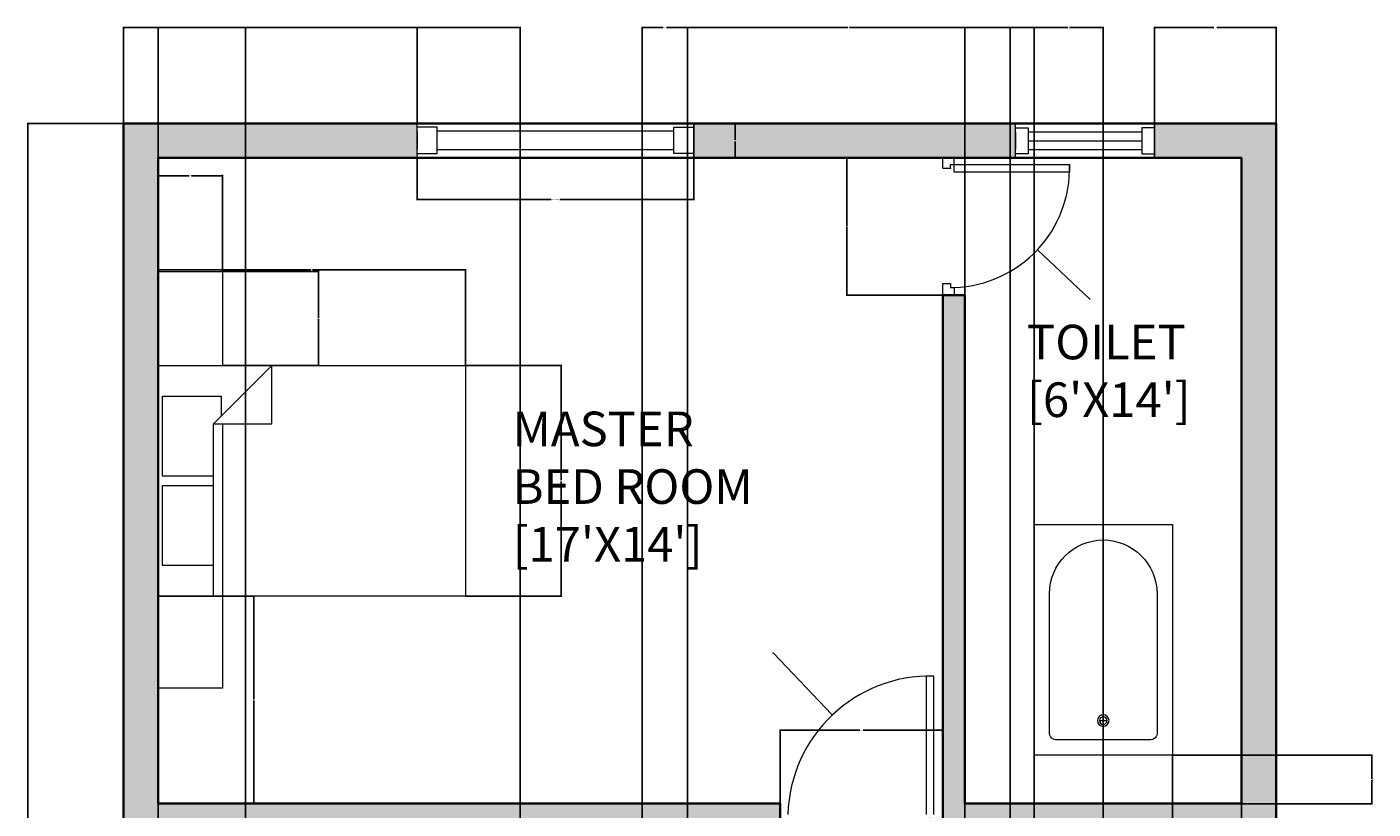
# Model space of a CAD drawing. Units: inches. Extents: x 2203 to 2554, y 381 to 929.
# Tile 3 of 3: x 2203 to 2554, y 726 to 929. Entities that reach past the tile are written whole.
import ezdxf

# ---------------------------------------------------------------- set-up
doc = ezdxf.new("R2010")
doc.units = ezdxf.units.IN
for name, color, linetype, lineweight in [('A-ANNO-DIMS', 2, 'Continuous', 18), ('A-AREA-IDEN', 7, 'Continuous', 18), ('A-DOOR', 239, 'Continuous', 18), ('A-FLOR-FIXT', 8, 'Continuous', 18), ('A-FURN', 8, 'Continuous', 18), ('A-GLAZ', 4, 'Continuous', 18), ('A-WALL', 7, 'Continuous', 35), ('A-WALL-PATT', 250, 'Continuous', 13)]:
    doc.layers.add(name, color=color, linetype=linetype, lineweight=lineweight)
doc.styles.get("Standard").update_dxf_attribs({"font": 'arial.ttf'})
doc.dimstyles.get("Standard").update_dxf_attribs({"dimtxt": 0.18, "dimasz": 0.18, "dimexe": 0.18, "dimexo": 0.0625, "dimgap": 0.09, "dimtad": 0, "dimtih": 1, "dimtoh": 1, "dimdec": 4, "dimzin": 0, "dimdsep": 46, "dimtxsty": 'Standard', "dimcen": 0.09, "dimadec": 0, "dimazin": 0, "dimtfac": 1, "dimtdec": 4, "dimtofl": 0, "dimtmove": 0, "dimatfit": 3, "dimfxl": 1, "dimtolj": 1, "dimtzin": 0, "dimarcsym": 0})

# ---------------------------------------------------------------- blocks, each defined once
blk = doc.blocks.new('WIN-36')
for p, q in [((0, 36.19), (9, 36.19)), ((0, 0), (0, 36.19)), ((0, 36.19), (4.5, 36.19)), ((1.12, 32.87), (1.12, 36.19)), ((6.76, 36.19), (2.25, 36.19)), ((7.88, 36.19), (7.88, 32.87)), ((9, 36.19), (9, 0)), ((7.88, 32.87), (1.12, 32.87)), ((2.25, 32.87), (2.25, 3.32)), ((4.5, 32.87), (4.5, 3.32)), ((6.76, 3.32), (6.76, 32.87)), ((9, 0), (0, 0)), ((2.25, 0), (0, 0)), ((0, 0), (6.76, 0)), ((7.88, 3.32), (1.12, 3.32)), ((1.12, 3.32), (1.12, 0)), ((4.5, 0), (6.76, 0)), ((6.76, 0), (9, 0)), ((7.88, 0), (7.88, 3.32))]:
    blk.add_line(p, q)
blk = doc.blocks.new('WIN-72')
for p, q in [((0, 0), (0, 9)), ((0, 9), (72, 9)), ((5.2, 7.99), (0, 7.99)), ((5.2, 1.13), (5.2, 7.99)), ((66.8, 1.13), (66.8, 7.99)), ((66.8, 7.99), (72, 7.99)), ((72, 9), (72, 0)), ((72, 6.99), (72, 9)), ((0, 6.99), (0, 2.25)), ((0, 0), (0, 4.5)), ((66.8, 6.99), (5.2, 6.99)), ((72, 4.5), (72, 6.99)), ((72, 2.25), (72, 6.99)), ((0, 1.13), (5.2, 1.13)), ((72, 0), (0, 0)), ((5.2, 2.25), (66.8, 2.25)), ((72, 1.13), (66.8, 1.13)), ((72, 0), (72, 2.25))]:
    blk.add_line(p, q)
blk = doc.blocks.new('TUB-36X60')
for p, q in [((17, 51), (19, 51)), ((18, 52), (18, 50))]:
    blk.add_line(p, q)
blk.add_lwpolyline([(36, 60), (0, 60), (0, 0), (36, 0)], close=True)
for points in [[(4, 54), (4, 18)], [(30, 56), (6, 56)], [(32, 18), (32, 54)]]:
    blk.add_lwpolyline(points)
for radius in [1.5, 1]:
    blk.add_circle((18, 51), radius)
for centre, radius, start, end in [((5.75, 54.25), 1.77, 81.8699, 188.1301), ((30.25, 54.25), 1.77, 351.8699, 98.1301), ((18, 18), 14, 180, 0)]:
    blk.add_arc(centre, radius, start, end)
blk = doc.blocks.new('*D15')
at = {"layer": 'A-ANNO-DIMS', "color": 0, "lineweight": -2, "transparency": 16777216}
for p, q in [((2305.03, 895), (2305.03, 884.08)), ((2377.03, 895), (2377.03, 884.08)), ((2305.21, 884.26), (2339.91, 884.26)), ((2376.85, 884.26), (2342.15, 884.26))]:
    blk.add_line(p, q, dxfattribs=at)
at = {"layer": 'A-ANNO-DIMS', "color": 0, "transparency": 16777216}
for points in [[(2305.21, 884.29), (2305.21, 884.23), (2305.03, 884.26)], [(2376.85, 884.29), (2376.85, 884.23), (2377.03, 884.26)]]:
    blk.add_solid(points, dxfattribs=at)
at = {"layer": 'Defpoints', "color": 0, "transparency": 16777216}
for p in [(2305.03, 895.06), (2377.03, 895.06), (2377.03, 884.26)]:
    blk.add_point(p, dxfattribs=at)
at = {"layer": 'A-ANNO-DIMS', "color": 0, "transparency": 16777216, "insert": (2341.03, 884.26), "char_height": 0.18, "attachment_point": 5}
blk.add_mtext('\\A1;WINDOW 72 TYP.', dxfattribs=at)
blk = doc.blocks.new('*D16')
at = {"layer": 'A-ANNO-DIMS', "color": 0, "lineweight": -2, "transparency": 16777216}
for p, q in [((2377.09, 904.06), (2388.01, 904.06)), ((2387.83, 903.88), (2387.83, 899.75)), ((2387.83, 895.24), (2387.83, 899.38)), ((2377.09, 895.06), (2388.01, 895.06))]:
    blk.add_line(p, q, dxfattribs=at)
at = {"layer": 'A-ANNO-DIMS', "color": 0, "transparency": 16777216}
for points in [[(2387.8, 903.88), (2387.86, 903.88), (2387.83, 904.06)], [(2387.8, 895.24), (2387.86, 895.24), (2387.83, 895.06)]]:
    blk.add_solid(points, dxfattribs=at)
at = {"layer": 'Defpoints', "color": 0, "transparency": 16777216}
for p in [(2377.03, 904.06), (2387.83, 904.06), (2377.03, 895.06)]:
    blk.add_point(p, dxfattribs=at)
at = {"layer": 'A-ANNO-DIMS', "color": 0, "transparency": 16777216, "insert": (2387.83, 899.56), "char_height": 0.18, "attachment_point": 5}
blk.add_mtext('\\A1;9 TYP.', dxfattribs=at)
blk = doc.blocks.new('*D22')
at = {"layer": 'A-ANNO-DIMS', "color": 0, "lineweight": -2, "transparency": 16777216}
for p, q in [((2228.54, 904.06), (2203.5, 904.06)), ((2203.68, 903.88), (2203.68, 655.25)), ((2203.68, 406.24), (2203.68, 654.88)), ((2228.54, 406.06), (2203.5, 406.06))]:
    blk.add_line(p, q, dxfattribs=at)
at = {"layer": 'A-ANNO-DIMS', "color": 0, "transparency": 16777216}
for points in [[(2203.65, 903.88), (2203.71, 903.88), (2203.68, 904.06)], [(2203.65, 406.24), (2203.71, 406.24), (2203.68, 406.06)]]:
    blk.add_solid(points, dxfattribs=at)
at = {"layer": 'Defpoints', "color": 0, "transparency": 16777216}
for p in [(2203.68, 904.06), (2228.6, 904.06), (2228.6, 406.06)]:
    blk.add_point(p, dxfattribs=at)
at = {"layer": 'A-ANNO-DIMS', "color": 0, "transparency": 16777216, "insert": (2203.68, 655.06), "char_height": 0.18, "attachment_point": 5}
blk.add_mtext('\\A1;498', dxfattribs=at)
blk = doc.blocks.new('*D23')
at = {"layer": 'A-ANNO-DIMS', "color": 0, "lineweight": -2, "transparency": 16777216}
for p, q in [((2228.6, 904.13), (2228.6, 929.16)), ((2228.78, 928.98), (2266.42, 928.98)), ((2304.85, 928.98), (2267.21, 928.98)), ((2305.03, 904.13), (2305.03, 929.16))]:
    blk.add_line(p, q, dxfattribs=at)
at = {"layer": 'A-ANNO-DIMS', "color": 0, "transparency": 16777216}
for points in [[(2228.78, 929.01), (2228.78, 928.95), (2228.6, 928.98)], [(2304.85, 929.01), (2304.85, 928.95), (2305.03, 928.98)]]:
    blk.add_solid(points, dxfattribs=at)
at = {"layer": 'Defpoints', "color": 0, "transparency": 16777216}
for p in [(2305.03, 928.98), (2228.6, 904.06), (2305.03, 904.06)]:
    blk.add_point(p, dxfattribs=at)
at = {"layer": 'A-ANNO-DIMS', "color": 0, "transparency": 16777216, "insert": (2266.81, 928.98), "char_height": 0.18, "attachment_point": 5}
blk.add_mtext('\\A1;76.43', dxfattribs=at)
blk = doc.blocks.new('*D24')
at = {"layer": 'A-ANNO-DIMS', "color": 0, "lineweight": -2, "transparency": 16777216}
for p, q in [((2496.97, 904.13), (2496.97, 929.16)), ((2497.15, 928.98), (2512.39, 928.98)), ((2528.42, 928.98), (2513.18, 928.98)), ((2528.6, 904.13), (2528.6, 929.16))]:
    blk.add_line(p, q, dxfattribs=at)
at = {"layer": 'A-ANNO-DIMS', "color": 0, "transparency": 16777216}
for points in [[(2497.15, 929.01), (2497.15, 928.95), (2496.97, 928.98)], [(2528.42, 929.01), (2528.42, 928.95), (2528.6, 928.98)]]:
    blk.add_solid(points, dxfattribs=at)
at = {"layer": 'Defpoints', "color": 0, "transparency": 16777216}
for p in [(2528.6, 928.98), (2496.97, 904.06), (2528.6, 904.06)]:
    blk.add_point(p, dxfattribs=at)
at = {"layer": 'A-ANNO-DIMS', "color": 0, "transparency": 16777216, "insert": (2512.78, 928.98), "char_height": 0.18, "attachment_point": 5}
blk.add_mtext('\\A1;31.63', dxfattribs=at)
blk = doc.blocks.new('*D30')
at = {"layer": 'A-ANNO-DIMS', "color": 0, "lineweight": -2, "transparency": 16777216}
for p, q in [((2237.6, 601.13), (2237.6, 929.16)), ((2237.78, 928.98), (2248.57, 928.98)), ((2260.15, 928.98), (2249.36, 928.98)), ((2260.33, 601.13), (2260.33, 929.16))]:
    blk.add_line(p, q, dxfattribs=at)
at = {"layer": 'A-ANNO-DIMS', "color": 0, "transparency": 16777216}
for points in [[(2237.78, 929.01), (2237.78, 928.95), (2237.6, 928.98)], [(2260.15, 929.01), (2260.15, 928.95), (2260.33, 928.98)]]:
    blk.add_solid(points, dxfattribs=at)
at = {"layer": 'Defpoints', "color": 0, "transparency": 16777216}
for p in [(2260.33, 928.98), (2237.6, 601.06), (2260.33, 601.06)]:
    blk.add_point(p, dxfattribs=at)
at = {"layer": 'A-ANNO-DIMS', "color": 0, "transparency": 16777216, "insert": (2248.96, 928.98), "char_height": 0.18, "attachment_point": 5}
blk.add_mtext('\\A1;22.73', dxfattribs=at)
blk = doc.blocks.new('*D31')
at = {"layer": 'A-ANNO-DIMS', "color": 0, "lineweight": -2, "transparency": 16777216}
for p, q in [((2260.33, 601.13), (2260.33, 929.16)), ((2260.51, 928.98), (2295.75, 928.98)), ((2331.64, 928.98), (2296.4, 928.98)), ((2331.82, 601.13), (2331.82, 929.16))]:
    blk.add_line(p, q, dxfattribs=at)
at = {"layer": 'A-ANNO-DIMS', "color": 0, "transparency": 16777216}
for points in [[(2260.51, 929.01), (2260.51, 928.95), (2260.33, 928.98)], [(2331.64, 929.01), (2331.64, 928.95), (2331.82, 928.98)]]:
    blk.add_solid(points, dxfattribs=at)
at = {"layer": 'Defpoints', "color": 0, "transparency": 16777216}
for p in [(2331.82, 928.98), (2260.33, 601.06), (2331.82, 601.06)]:
    blk.add_point(p, dxfattribs=at)
at = {"layer": 'A-ANNO-DIMS', "color": 0, "transparency": 16777216, "insert": (2296.08, 928.98), "char_height": 0.18, "attachment_point": 5}
blk.add_mtext('\\A1;71.5', dxfattribs=at)
blk = doc.blocks.new('*D35')
at = {"layer": 'A-ANNO-DIMS', "color": 0, "lineweight": -2, "transparency": 16777216}
for p, q in [((2399.53, 721.31), (2399.53, 746.34)), ((2441.82, 721.31), (2441.82, 746.34)), ((2399.71, 746.16), (2420.28, 746.16)), ((2441.64, 746.16), (2421.08, 746.16))]:
    blk.add_line(p, q, dxfattribs=at)
at = {"layer": 'A-ANNO-DIMS', "color": 0, "transparency": 16777216}
for points in [[(2399.71, 746.19), (2399.71, 746.13), (2399.53, 746.16)], [(2441.64, 746.19), (2441.64, 746.13), (2441.82, 746.16)]]:
    blk.add_solid(points, dxfattribs=at)
at = {"layer": 'Defpoints', "color": 0, "transparency": 16777216}
for p in [(2441.82, 746.16), (2399.53, 721.24), (2441.82, 721.24)]:
    blk.add_point(p, dxfattribs=at)
at = {"layer": 'A-ANNO-DIMS', "color": 0, "transparency": 16777216, "insert": (2420.68, 746.16), "char_height": 0.18, "attachment_point": 5}
blk.add_mtext('\\A1;42.29', dxfattribs=at)
blk = doc.blocks.new('*D36')
at = {"layer": 'A-ANNO-DIMS', "color": 0, "lineweight": -2, "transparency": 16777216}
for p, q in [((2441.76, 895.06), (2416.72, 895.06)), ((2416.9, 894.88), (2416.9, 877.41)), ((2416.9, 859.57), (2416.9, 877.04)), ((2441.76, 859.39), (2416.72, 859.39))]:
    blk.add_line(p, q, dxfattribs=at)
at = {"layer": 'A-ANNO-DIMS', "color": 0, "transparency": 16777216}
for points in [[(2416.87, 894.88), (2416.93, 894.88), (2416.9, 895.06)], [(2416.87, 859.57), (2416.93, 859.57), (2416.9, 859.39)]]:
    blk.add_solid(points, dxfattribs=at)
at = {"layer": 'Defpoints', "color": 0, "transparency": 16777216}
for p in [(2416.9, 895.06), (2441.82, 895.06), (2441.82, 859.39)]:
    blk.add_point(p, dxfattribs=at)
at = {"layer": 'A-ANNO-DIMS', "color": 0, "transparency": 16777216, "insert": (2416.9, 877.23), "char_height": 0.18, "attachment_point": 5}
blk.add_mtext('\\A1;35.68', dxfattribs=at)
blk = doc.blocks.new('*D38')
at = {"layer": 'A-ANNO-DIMS', "color": 0, "lineweight": -2, "transparency": 16777216}
for p, q in [((2237.6, 841.13), (2237.6, 866.16)), ((2237.78, 865.98), (2277.38, 865.98)), ((2317.42, 865.98), (2277.82, 865.98)), ((2317.6, 841.13), (2317.6, 866.16))]:
    blk.add_line(p, q, dxfattribs=at)
at = {"layer": 'A-ANNO-DIMS', "color": 0, "transparency": 16777216}
for points in [[(2237.78, 866.01), (2237.78, 865.95), (2237.6, 865.98)], [(2317.42, 866.01), (2317.42, 865.95), (2317.6, 865.98)]]:
    blk.add_solid(points, dxfattribs=at)
at = {"layer": 'Defpoints', "color": 0, "transparency": 16777216}
for p in [(2317.6, 865.98), (2237.6, 841.06), (2317.6, 841.06)]:
    blk.add_point(p, dxfattribs=at)
at = {"layer": 'A-ANNO-DIMS', "color": 0, "transparency": 16777216, "insert": (2277.6, 865.98), "char_height": 0.18, "attachment_point": 5}
blk.add_mtext('\\A1;80', dxfattribs=at)
blk = doc.blocks.new('*D39')
at = {"layer": 'A-ANNO-DIMS', "color": 0, "lineweight": -2, "transparency": 16777216}
for p, q in [((2317.66, 841.06), (2342.7, 841.06)), ((2342.52, 840.88), (2342.52, 811.25)), ((2342.52, 781.24), (2342.52, 810.88)), ((2317.66, 781.06), (2342.7, 781.06))]:
    blk.add_line(p, q, dxfattribs=at)
at = {"layer": 'A-ANNO-DIMS', "color": 0, "transparency": 16777216}
for points in [[(2342.49, 840.88), (2342.55, 840.88), (2342.52, 841.06)], [(2342.49, 781.24), (2342.55, 781.24), (2342.52, 781.06)]]:
    blk.add_solid(points, dxfattribs=at)
at = {"layer": 'Defpoints', "color": 0, "transparency": 16777216}
for p in [(2317.6, 841.06), (2317.6, 781.06), (2342.52, 781.06)]:
    blk.add_point(p, dxfattribs=at)
at = {"layer": 'A-ANNO-DIMS', "color": 0, "transparency": 16777216, "insert": (2342.52, 811.06), "char_height": 0.18, "attachment_point": 5}
blk.add_mtext('\\A1;60', dxfattribs=at)
blk = doc.blocks.new('*D40')
at = {"layer": 'A-ANNO-DIMS', "color": 0, "lineweight": -2, "transparency": 16777216}
for p, q in [((2237.66, 781.06), (2262.7, 781.06)), ((2262.52, 780.88), (2262.52, 754.25)), ((2262.52, 727.24), (2262.52, 753.88)), ((2237.66, 727.06), (2262.7, 727.06))]:
    blk.add_line(p, q, dxfattribs=at)
at = {"layer": 'A-ANNO-DIMS', "color": 0, "transparency": 16777216}
for points in [[(2262.49, 780.88), (2262.55, 780.88), (2262.52, 781.06)], [(2262.49, 727.24), (2262.55, 727.24), (2262.52, 727.06)]]:
    blk.add_solid(points, dxfattribs=at)
at = {"layer": 'Defpoints', "color": 0, "transparency": 16777216}
for p in [(2237.6, 781.06), (2237.6, 727.06), (2262.52, 727.06)]:
    blk.add_point(p, dxfattribs=at)
at = {"layer": 'A-ANNO-DIMS', "color": 0, "transparency": 16777216, "insert": (2262.52, 754.06), "char_height": 0.18, "attachment_point": 5}
blk.add_mtext('\\A1;54', dxfattribs=at)
blk = doc.blocks.new('*D41')
at = {"layer": 'A-ANNO-DIMS', "color": 0, "lineweight": -2, "transparency": 16777216}
for p, q in [((2375.37, 509.13), (2375.37, 929.16)), ((2375.55, 928.98), (2417.15, 928.98)), ((2459.19, 928.98), (2417.59, 928.98)), ((2459.37, 509.13), (2459.37, 929.16))]:
    blk.add_line(p, q, dxfattribs=at)
at = {"layer": 'A-ANNO-DIMS', "color": 0, "transparency": 16777216}
for points in [[(2375.55, 929.01), (2375.55, 928.95), (2375.37, 928.98)], [(2459.19, 929.01), (2459.19, 928.95), (2459.37, 928.98)]]:
    blk.add_solid(points, dxfattribs=at)
at = {"layer": 'Defpoints', "color": 0, "transparency": 16777216}
for p in [(2459.37, 928.98), (2375.37, 509.06), (2459.37, 509.06)]:
    blk.add_point(p, dxfattribs=at)
at = {"layer": 'A-ANNO-DIMS', "color": 0, "transparency": 16777216, "insert": (2417.37, 928.98), "char_height": 0.18, "attachment_point": 5}
blk.add_mtext('\\A1;84', dxfattribs=at)
blk = doc.blocks.new('*D43')
at = {"layer": 'A-ANNO-DIMS', "color": 0, "lineweight": -2, "transparency": 16777216}
for p, q in [((2363.6, 500.21), (2363.6, 929.16)), ((2363.78, 928.98), (2369.03, 928.98)), ((2375.19, 928.98), (2369.94, 928.98)), ((2375.37, 509.13), (2375.37, 929.16))]:
    blk.add_line(p, q, dxfattribs=at)
at = {"layer": 'A-ANNO-DIMS', "color": 0, "transparency": 16777216}
for points in [[(2363.78, 929.01), (2363.78, 928.95), (2363.6, 928.98)], [(2375.19, 929.01), (2375.19, 928.95), (2375.37, 928.98)]]:
    blk.add_solid(points, dxfattribs=at)
at = {"layer": 'Defpoints', "color": 0, "transparency": 16777216}
for p in [(2375.37, 928.98), (2375.37, 509.06), (2363.6, 500.15)]:
    blk.add_point(p, dxfattribs=at)
at = {"layer": 'A-ANNO-DIMS', "color": 0, "transparency": 16777216, "insert": (2369.49, 928.98), "char_height": 0.18, "attachment_point": 5}
blk.add_mtext('\\A1;11.775', dxfattribs=at)
blk = doc.blocks.new('*D50')
at = {"layer": 'A-ANNO-DIMS', "color": 0, "lineweight": -2, "transparency": 16777216}
for p, q in [((2465.6, 707.5), (2465.6, 929.16)), ((2465.78, 928.98), (2474.39, 928.98)), ((2483.42, 928.98), (2474.81, 928.98)), ((2483.6, 698.5), (2483.6, 929.16))]:
    blk.add_line(p, q, dxfattribs=at)
at = {"layer": 'A-ANNO-DIMS', "color": 0, "transparency": 16777216}
for points in [[(2465.78, 929.01), (2465.78, 928.95), (2465.6, 928.98)], [(2483.42, 929.01), (2483.42, 928.95), (2483.6, 928.98)]]:
    blk.add_solid(points, dxfattribs=at)
at = {"layer": 'Defpoints', "color": 0, "transparency": 16777216}
for p in [(2483.6, 928.98), (2465.6, 707.44), (2483.6, 698.44)]:
    blk.add_point(p, dxfattribs=at)
at = {"layer": 'A-ANNO-DIMS', "color": 0, "transparency": 16777216, "insert": (2474.6, 928.98), "char_height": 0.18, "attachment_point": 5}
blk.add_mtext('\\A1;18', dxfattribs=at)
blk = doc.blocks.new('*D52')
at = {"layer": 'A-ANNO-DIMS', "color": 0, "lineweight": -2, "transparency": 16777216}
for p, q in [((2447.6, 721.31), (2447.6, 929.16)), ((2447.78, 928.98), (2456.39, 928.98)), ((2465.42, 928.98), (2456.81, 928.98)), ((2465.6, 707.5), (2465.6, 929.16))]:
    blk.add_line(p, q, dxfattribs=at)
at = {"layer": 'A-ANNO-DIMS', "color": 0, "transparency": 16777216}
for points in [[(2447.78, 929.01), (2447.78, 928.95), (2447.6, 928.98)], [(2465.42, 929.01), (2465.42, 928.95), (2465.6, 928.98)]]:
    blk.add_solid(points, dxfattribs=at)
at = {"layer": 'Defpoints', "color": 0, "transparency": 16777216}
for p in [(2447.6, 928.98), (2447.6, 721.24), (2465.6, 707.44)]:
    blk.add_point(p, dxfattribs=at)
at = {"layer": 'A-ANNO-DIMS', "color": 0, "transparency": 16777216, "insert": (2456.6, 928.98), "char_height": 0.18, "attachment_point": 5}
blk.add_mtext('\\A1;18', dxfattribs=at)
blk = doc.blocks.new('*D54')
at = {"layer": 'A-ANNO-DIMS', "color": 0, "lineweight": -2, "transparency": 16777216}
for p, q in [((2501.66, 739.68), (2553.7, 739.68)), ((2553.52, 739.5), (2553.52, 733.55)), ((2553.52, 727.24), (2553.52, 733.19)), ((2519.66, 727.06), (2553.7, 727.06))]:
    blk.add_line(p, q, dxfattribs=at)
at = {"layer": 'A-ANNO-DIMS', "color": 0, "transparency": 16777216}
for points in [[(2553.49, 739.5), (2553.55, 739.5), (2553.52, 739.68)], [(2553.49, 727.24), (2553.55, 727.24), (2553.52, 727.06)]]:
    blk.add_solid(points, dxfattribs=at)
at = {"layer": 'Defpoints', "color": 0, "transparency": 16777216}
for p in [(2501.6, 739.68), (2519.6, 727.06), (2553.52, 727.06)]:
    blk.add_point(p, dxfattribs=at)
at = {"layer": 'A-ANNO-DIMS', "color": 0, "transparency": 16777216, "insert": (2553.52, 733.37), "char_height": 0.18, "attachment_point": 5}
blk.add_mtext('\\A1;12.61', dxfattribs=at)
blk = doc.blocks.new('*D55')
at = {"layer": 'A-ANNO-DIMS', "color": 0, "lineweight": -2, "transparency": 16777216}
for p, q in [((2501.6, 739.61), (2501.6, 380.96)), ((2519.6, 727), (2519.6, 380.96)), ((2501.78, 381.14), (2510.39, 381.14)), ((2519.42, 381.14), (2510.81, 381.14))]:
    blk.add_line(p, q, dxfattribs=at)
at = {"layer": 'A-ANNO-DIMS', "color": 0, "transparency": 16777216}
for points in [[(2501.78, 381.17), (2501.78, 381.11), (2501.6, 381.14)], [(2519.42, 381.17), (2519.42, 381.11), (2519.6, 381.14)]]:
    blk.add_solid(points, dxfattribs=at)
at = {"layer": 'Defpoints', "color": 0, "transparency": 16777216}
for p in [(2501.6, 739.68), (2519.6, 727.06), (2519.6, 381.14)]:
    blk.add_point(p, dxfattribs=at)
at = {"layer": 'A-ANNO-DIMS', "color": 0, "transparency": 16777216, "insert": (2510.6, 381.14), "char_height": 0.18, "attachment_point": 5}
blk.add_mtext('\\A1;18', dxfattribs=at)
blk = doc.blocks.new('*D58')
at = {"layer": 'A-ANNO-DIMS', "color": 0, "lineweight": -2, "transparency": 16777216}
for p, q in [((2237.6, 865.61), (2237.6, 890.64)), ((2237.78, 890.46), (2245.68, 890.46)), ((2254.22, 890.46), (2246.31, 890.46)), ((2254.4, 865.61), (2254.4, 890.64))]:
    blk.add_line(p, q, dxfattribs=at)
at = {"layer": 'A-ANNO-DIMS', "color": 0, "transparency": 16777216}
for points in [[(2237.78, 890.49), (2237.78, 890.43), (2237.6, 890.46)], [(2254.22, 890.49), (2254.22, 890.43), (2254.4, 890.46)]]:
    blk.add_solid(points, dxfattribs=at)
at = {"layer": 'Defpoints', "color": 0, "transparency": 16777216}
for p in [(2254.4, 890.46), (2237.6, 865.54), (2254.4, 865.54)]:
    blk.add_point(p, dxfattribs=at)
at = {"layer": 'A-ANNO-DIMS', "color": 0, "transparency": 16777216, "insert": (2246, 890.46), "char_height": 0.18, "attachment_point": 5}
blk.add_mtext('\\A1;16.8', dxfattribs=at)
blk = doc.blocks.new('*D59')
at = {"layer": 'A-ANNO-DIMS', "color": 0, "lineweight": -2, "transparency": 16777216}
for p, q in [((2254.46, 865.54), (2279.5, 865.54)), ((2279.32, 865.36), (2279.32, 853.49)), ((2279.32, 841.24), (2279.32, 853.12)), ((2254.46, 841.06), (2279.5, 841.06))]:
    blk.add_line(p, q, dxfattribs=at)
at = {"layer": 'A-ANNO-DIMS', "color": 0, "transparency": 16777216}
for points in [[(2279.29, 865.36), (2279.35, 865.36), (2279.32, 865.54)], [(2279.29, 841.24), (2279.35, 841.24), (2279.32, 841.06)]]:
    blk.add_solid(points, dxfattribs=at)
at = {"layer": 'Defpoints', "color": 0, "transparency": 16777216}
for p in [(2254.4, 865.54), (2254.4, 841.06), (2279.32, 841.06)]:
    blk.add_point(p, dxfattribs=at)
at = {"layer": 'A-ANNO-DIMS', "color": 0, "transparency": 16777216, "insert": (2279.32, 853.3), "char_height": 0.18, "attachment_point": 5}
blk.add_mtext('\\A1;24.48', dxfattribs=at)
blk = doc.blocks.new('*D63')
at = {"layer": 'A-ANNO-DIMS', "color": 0, "lineweight": -2, "transparency": 16777216}
for p, q in [((2397.62, 766.24), (2397.8, 766.24)), ((2397.8, 766.24), (2412.95, 750.24)), ((2438.44, 723.24), (2438.62, 723.24)), ((2438.53, 723.15), (2438.53, 723.33))]:
    blk.add_line(p, q, dxfattribs=at)
at = {"layer": 'A-ANNO-DIMS', "color": 0, "transparency": 16777216}
blk.add_solid([(2412.97, 750.27), (2412.93, 750.22), (2413.08, 750.11)], dxfattribs=at)
at = {"layer": 'Defpoints', "color": 0, "transparency": 16777216}
for p in [(2413.08, 750.11), (2438.53, 723.24)]:
    blk.add_point(p, dxfattribs=at)
at = {"layer": 'A-ANNO-DIMS', "color": 0, "transparency": 16777216, "insert": (2397.16, 766.24), "char_height": 0.18, "attachment_point": 5}
blk.add_mtext('\\A1;R37.01', dxfattribs=at)
blk = doc.blocks.new('*D64')
at = {"layer": 'A-ANNO-DIMS', "color": 0, "lineweight": -2, "transparency": 16777216}
for p, q in [((2443.73, 892.39), (2443.91, 892.39)), ((2443.82, 892.3), (2443.82, 892.48)), ((2480.03, 858.45), (2466.58, 871.05)), ((2480.21, 858.45), (2480.03, 858.45))]:
    blk.add_line(p, q, dxfattribs=at)
at = {"layer": 'A-ANNO-DIMS', "color": 0, "transparency": 16777216}
blk.add_solid([(2466.6, 871.07), (2466.56, 871.03), (2466.45, 871.17)], dxfattribs=at)
at = {"layer": 'Defpoints', "color": 0, "transparency": 16777216}
for p in [(2443.82, 892.39), (2466.45, 871.17)]:
    blk.add_point(p, dxfattribs=at)
at = {"layer": 'A-ANNO-DIMS', "color": 0, "transparency": 16777216, "insert": (2480.76, 858.45), "char_height": 0.18, "attachment_point": 5}
blk.add_mtext('\\A1;R31.016', dxfattribs=at)

msp = doc.modelspace()

# ---------------------------------------------------------------- hatches: boundary and pattern name
at = {"layer": 'A-WALL-PATT'}
h = msp.add_hatch(color=256, dxfattribs=at)
h.dxf.hatch_style = 1
h.paths.add_polyline_path([(2237.599, 595.0647), (2260.3281, 595.0647), (2260.3281, 601.0647), (2237.599, 601.0647), (2237.599, 621.2584), (2233.099, 621.2584), (2230.6109, 621.2584), (2228.599, 621.2584), (2228.599, 466.0647), (2261.0302, 466.0647), (2261.0302, 470.5647), (2261.0302, 473.0528), (2261.0302, 475.0647), (2237.599, 475.0647)])
h.paths.add_polyline_path([(2237.599, 895.0647), (2305.0273, 895.0647), (2305.0273, 899.5647), (2305.0273, 904.0647), (2228.599, 904.0647), (2228.599, 693.2584), (2230.6109, 693.2584), (2235.349, 693.2584), (2237.599, 693.2584), (2237.599, 721.2436), (2357.599, 721.2436), (2357.599, 601.0647), (2331.8237, 601.0647), (2331.8237, 595.0647), (2357.599, 595.0647), (2357.599, 570.3283), (2363.599, 570.3283), (2363.599, 595.0647), (2363.599, 601.0647), (2363.599, 721.2436), (2399.5308, 721.2436), (2399.5308, 724.2436), (2399.5308, 727.0647), (2237.599, 727.0647)])
h.paths.add_polyline_path([(2447.599, 859.3877), (2441.8244, 859.3877), (2441.8244, 727.0647), (2441.8244, 721.2436), (2441.8244, 691.5632), (2441.8244, 631.1686), (2444.8244, 631.1686), (2447.599, 631.1686), (2447.599, 721.2436), (2519.599, 721.2436), (2519.599, 691.5572), (2524.099, 691.5572), (2526.3564, 691.5572), (2528.599, 691.5572), (2528.599, 904.0647), (2496.9662, 904.0647), (2496.9662, 901.8221), (2496.9662, 895.0647), (2519.599, 895.0647), (2519.599, 727.0647), (2447.599, 727.0647)])
h.paths.add_polyline_path([(2460.78, 904.0647), (2377.0273, 904.0647), (2377.0273, 902.0528), (2377.0273, 895.0647), (2441.8244, 895.0647), (2460.78, 895.0647), (2460.78, 899.5647)])
h.paths.add_polyline_path([(2471.599, 475.0647), (2363.599, 475.0647), (2363.599, 500.1465), (2357.599, 500.1465), (2357.599, 475.0647), (2333.0302, 475.0647), (2333.0302, 473.0528), (2333.0302, 468.3147), (2333.0302, 466.0647), (2471.599, 466.0647), (2471.599, 469.0647)])

# ---------------------------------------------------------------- linework, layer by layer
at = {"layer": 'A-DOOR'}
for p, q in [((2444.8244, 895.0647), (2441.8244, 895.0647)), ((2441.8244, 892.3877), (2441.8244, 895.0647)), ((2444.8244, 893.3877), (2444.8244, 895.0647)), ((2441.8244, 892.3877), (2443.8244, 892.3877)), ((2443.8244, 892.3877), (2443.8244, 893.3877)), ((2443.8244, 893.3877), (2444.8244, 893.3877)), ((2444.8244, 893.3877), (2474.8244, 893.3877)), ((2444.8244, 891.3877), (2444.8244, 893.3877)), ((2474.8244, 891.3877), (2444.8244, 891.3877)), ((2474.8244, 893.3877), (2474.8244, 891.3877)), ((2441.8244, 859.3877), (2441.8244, 862.3877)), ((2441.8244, 862.3877), (2443.8244, 862.3877)), ((2441.8244, 859.3877), (2441.8244, 862.3877)), ((2441.8244, 859.3877), (2441.8244, 862.3877)), ((2443.8244, 862.3877), (2443.8244, 861.3877)), ((2444.8244, 859.3877), (2441.8244, 859.3877)), ((2443.8244, 861.3877), (2444.8244, 861.3877)), ((2444.8244, 861.3877), (2444.8244, 859.3877)), ((2439.5308, 760.2436), (2437.5308, 760.2436)), ((2437.5308, 760.2436), (2437.5308, 724.2436)), ((2439.5308, 724.2436), (2439.5308, 760.2436))]:
    msp.add_line(p, q, dxfattribs=at)
for centre, radius, start, end in [((2443.8244, 892.3877), 31.0161, 271.84761, 1.84761), ((2438.5308, 723.2436), 37.0135, 88.451842, 178.451842)]:
    msp.add_arc(centre, radius, start, end, dxfattribs=at)
at = {"layer": 'A-FURN'}
for p, q in [((2237.599, 841.0647), (2237.599, 865.5438)), ((2237.599, 865.5438), (2254.399, 865.5438)), ((2254.399, 865.5438), (2254.399, 841.0647)), ((2237.599, 781.0647), (2237.599, 841.0647)), ((2237.599, 841.0647), (2317.599, 841.0647)), ((2237.599, 757.0749), (2237.599, 841.0647)), ((2267.199, 841.0647), (2251.999, 825.8647)), ((2267.199, 825.8647), (2267.199, 841.0647)), ((2317.599, 841.0647), (2317.599, 781.0647)), ((2238.799, 833.0647), (2253.999, 833.0647)), ((2238.799, 812.2647), (2238.799, 833.0647)), ((2253.999, 833.0647), (2253.999, 827.8641)), ((2251.999, 781.0647), (2251.999, 825.8647)), ((2251.999, 825.8647), (2267.199, 825.8647)), ((2254.399, 825.8647), (2254.399, 781.0647)), ((2251.999, 812.2647), (2238.799, 812.2647)), ((2238.799, 809.8647), (2251.999, 809.8647)), ((2238.799, 789.0647), (2238.799, 809.8647)), ((2251.999, 789.0647), (2238.799, 789.0647)), ((2317.599, 781.0647), (2237.599, 781.0647)), ((2254.399, 781.0647), (2254.399, 757.0749)), ((2254.399, 757.0749), (2237.599, 757.0749))]:
    msp.add_line(p, q, dxfattribs=at)
at = {"layer": 'A-WALL'}
for p, q in [((2228.599, 904.0647), (2528.599, 904.0647)), ((2228.599, 466.0647), (2228.599, 904.0647)), ((2528.599, 904.0647), (2459.599, 904.0647)), ((2528.599, 904.0647), (2528.599, 466.0647)), ((2528.599, 466.0647), (2528.599, 904.0647)), ((2237.599, 895.0647), (2519.599, 895.0647)), ((2237.599, 895.0647), (2441.8244, 895.0647)), ((2237.599, 727.0647), (2237.599, 895.0647)), ((2237.599, 727.0647), (2237.599, 895.0647)), ((2519.599, 895.0647), (2447.599, 895.0647)), ((2519.599, 895.0647), (2519.599, 727.0647)), ((2441.8244, 859.3877), (2441.8244, 727.0647)), ((2441.8244, 859.3877), (2447.599, 859.3877)), ((2447.599, 859.3877), (2447.599, 727.0647)), ((2399.5308, 727.0647), (2237.599, 727.0647)), ((2399.5308, 721.2436), (2399.5308, 727.0647)), ((2441.8244, 727.0647), (2441.8244, 721.2436)), ((2447.599, 727.0647), (2519.599, 727.0647))]:
    msp.add_line(p, q, dxfattribs=at)

# ---------------------------------------------------------------- block references
at = {"layer": 'A-FLOR-FIXT', "extrusion": (0, 0, -1), "zscale": -1, "rotation": 180}
msp.add_blockref('TUB-36X60', (-2465.599, 799.6759), dxfattribs=at)
at = {"layer": 'A-GLAZ'}
msp.add_blockref('WIN-72', (2305.0273, 895.0647), dxfattribs=at)
at = {"layer": 'A-GLAZ', "rotation": 90}
msp.add_blockref('WIN-36', (2496.9662, 895.0647), dxfattribs=at)

# ---------------------------------------------------------------- texts
at = {"layer": 'A-AREA-IDEN', "char_height": 9, "attachment_point": 1}
for s, insert in [("TOILET\\P[6'X14']", (2463.7556, 851.6717)), ("MASTER\\PBED ROOM\\P[17'X14']", (2329.8746, 829.0744))]:
    msp.add_mtext_dynamic_manual_height_columns(s, width=83.503544, gutter_width=12.5, heights=[0], dxfattribs=dict(at, insert=insert))

# ---------------------------------------------------------------- dimensions: what is measured, and where the dimension line sits
at = {"layer": 'A-ANNO-DIMS'}
for base, p1, p2, override, picture, middle in [((2305.0273, 928.9847), (2228.599, 904.0647), (2305.0273, 904.0647), {"dimdec": 2, "dimlfac": 1, "dimrnd": 0, "dimzin": 0, "dimdsep": 46, "dimlunit": 2}, '*D23', (2266.8131, 928.9847)), ((2260.3281, 928.9847), (2237.599, 601.0647), (2260.3281, 601.0647), {"dimdec": 2, "dimlfac": 1, "dimrnd": 0, "dimzin": 0, "dimdsep": 46, "dimlunit": 2}, '*D30', (2248.9636, 928.9847)), ((2331.8237, 928.9847), (2260.3281, 601.0647), (2331.8237, 601.0647), {"dimdec": 1, "dimlfac": 1, "dimrnd": 0, "dimzin": 0, "dimdsep": 46, "dimlunit": 2}, '*D31', (2296.0759, 928.9847)), ((2375.3736, 928.9847), (2363.599, 500.1465), (2375.3736, 509.0647), {"dimdec": 3, "dimlfac": 1, "dimrnd": 0, "dimzin": 0, "dimdsep": 46, "dimlunit": 2}, '*D43', (2369.4863, 928.9847)), ((2459.3736, 928.9847), (2375.3736, 509.0647), (2459.3736, 509.0647), {"dimdec": 0, "dimlfac": 1, "dimrnd": 0, "dimzin": 0, "dimdsep": 46, "dimlunit": 2}, '*D41', (2417.3736, 928.9847)), ((2447.599, 928.9847), (2465.599, 707.4353), (2447.599, 721.2436), {"dimdec": 0, "dimlfac": 1, "dimrnd": 0, "dimzin": 0, "dimdsep": 46, "dimlunit": 2}, '*D52', (2456.599, 928.9847)), ((2483.599, 928.9847), (2465.599, 707.4353), (2483.599, 698.4353), {"dimdec": 0, "dimlfac": 1, "dimrnd": 0, "dimzin": 0, "dimdsep": 46, "dimlunit": 2}, '*D50', (2474.599, 928.9847)), ((2528.599, 928.9847), (2496.9662, 904.0647), (2528.599, 904.0647), {"dimdec": 2, "dimlfac": 1, "dimrnd": 0, "dimzin": 0, "dimdsep": 46, "dimlunit": 2}, '*D24', (2512.7826, 928.9847)), ((2254.399, 890.4638), (2237.599, 865.5438), (2254.399, 865.5438), {"dimdec": 1, "dimlfac": 1, "dimrnd": 0, "dimzin": 0, "dimdsep": 46, "dimlunit": 2}, '*D58', (2245.999, 890.4638)), ((2317.599, 865.9847), (2237.599, 841.0647), (2317.599, 841.0647), {"dimdec": 0, "dimlfac": 1, "dimrnd": 0, "dimzin": 0, "dimdsep": 46, "dimlunit": 2}, '*D38', (2277.599, 865.9847)), ((2441.8244, 746.1636), (2399.5308, 721.2436), (2441.8244, 721.2436), {"dimdec": 2, "dimlfac": 1, "dimrnd": 0, "dimzin": 0, "dimdsep": 46, "dimlunit": 2}, '*D35', (2420.6776, 746.1636)), ((2519.599, 381.1447), (2501.599, 739.6759), (2519.599, 727.0647), {"dimdec": 0, "dimlfac": 1, "dimrnd": 0, "dimzin": 0, "dimdsep": 46, "dimlunit": 2}, '*D55', (2510.599, 381.1447))]:
    dim = msp.add_linear_dim(base=base, p1=p1, p2=p2, dimstyle='Standard', override=override, dxfattribs=at)
    dim.commit()
    dim.dimension.update_dxf_attribs({"geometry": picture, "text_midpoint": middle})
for base, p1, p2, angle, override, picture, middle in [((2203.679, 904.0647), (2228.599, 406.0647), (2228.599, 904.0647), 90, {"dimdec": 0, "dimlfac": 1, "dimrnd": 0, "dimzin": 0, "dimdsep": 46, "dimlunit": 2}, '*D22', (2203.679, 655.0647)), ((2416.9044, 895.0647), (2441.8244, 859.3877), (2441.8244, 895.0647), 90, {"dimdec": 2, "dimlfac": 1, "dimrnd": 0, "dimzin": 0, "dimdsep": 46, "dimlunit": 2}, '*D36', (2416.9044, 877.2262)), ((2279.319, 841.0647), (2254.399, 865.5438), (2254.399, 841.0647), 270, {"dimdec": 2, "dimlfac": 1, "dimrnd": 0, "dimzin": 0, "dimdsep": 46, "dimlunit": 2}, '*D59', (2279.319, 853.3042)), ((2342.519, 781.0647), (2317.599, 841.0647), (2317.599, 781.0647), 270, {"dimdec": 0, "dimlfac": 1, "dimrnd": 0, "dimzin": 0, "dimdsep": 46, "dimlunit": 2}, '*D39', (2342.519, 811.0647)), ((2262.519, 727.0647), (2237.599, 781.0647), (2237.599, 727.0647), 270, {"dimdec": 0, "dimlfac": 1, "dimrnd": 0, "dimzin": 0, "dimdsep": 46, "dimlunit": 2}, '*D40', (2262.519, 754.0647)), ((2553.519, 727.0647), (2501.599, 739.6759), (2519.599, 727.0647), 90, {"dimdec": 2, "dimlfac": 1, "dimrnd": 0, "dimzin": 0, "dimdsep": 46, "dimlunit": 2}, '*D54', (2553.519, 733.3703))]:
    dim = msp.add_linear_dim(base=base, p1=p1, p2=p2, angle=angle, dimstyle='Standard', override=override, dxfattribs=at)
    dim.commit()
    dim.dimension.update_dxf_attribs({"geometry": picture, "text_midpoint": middle})
dim = msp.add_linear_dim(base=(2387.8273, 904.0647), p1=(2377.0273, 895.0647), p2=(2377.0273, 904.0647), angle=90, text='<> TYP.', dimstyle='Standard', override={"dimdec": 0, "dimlfac": 1, "dimrnd": 0, "dimzin": 0, "dimdsep": 46, "dimlunit": 2}, dxfattribs=at)
dim.commit()
dim.dimension.update_dxf_attribs({"geometry": '*D16', "text_midpoint": (2387.8273, 899.5647)})
dim = msp.add_linear_dim(base=(2377.0273, 884.2647), p1=(2305.0273, 895.0647), p2=(2377.0273, 895.0647), text='WINDOW <> TYP.', dimstyle='Standard', override={"dimdec": 0, "dimlfac": 1, "dimrnd": 0, "dimzin": 0, "dimdsep": 46, "dimlunit": 2}, dxfattribs=at)
dim.commit()
dim.dimension.update_dxf_attribs({"geometry": '*D15', "text_midpoint": (2341.0273, 884.2647)})
for center, mpoint, override, picture, middle in [((2443.8244, 892.3877), (2466.4517, 871.1743), {"dimdec": 3, "dimlfac": 1, "dimrnd": 0, "dimzin": 0, "dimdsep": 46, "dimlunit": 2}, '*D64', (2480.7577, 858.4463)), ((2438.5308, 723.2436), (2413.0751, 750.1138), {"dimdec": 2, "dimlfac": 1, "dimrnd": 0, "dimzin": 0, "dimdsep": 46, "dimlunit": 2}, '*D63', (2397.1593, 766.236))]:
    dim = msp.add_radius_dim(center=center, mpoint=mpoint, dimstyle='Standard', override=override, dxfattribs=at)
    dim.commit()
    dim.dimension.update_dxf_attribs({"geometry": picture, "text_midpoint": middle, "dimtype": 164})

doc.saveas('drawing.dxf')
